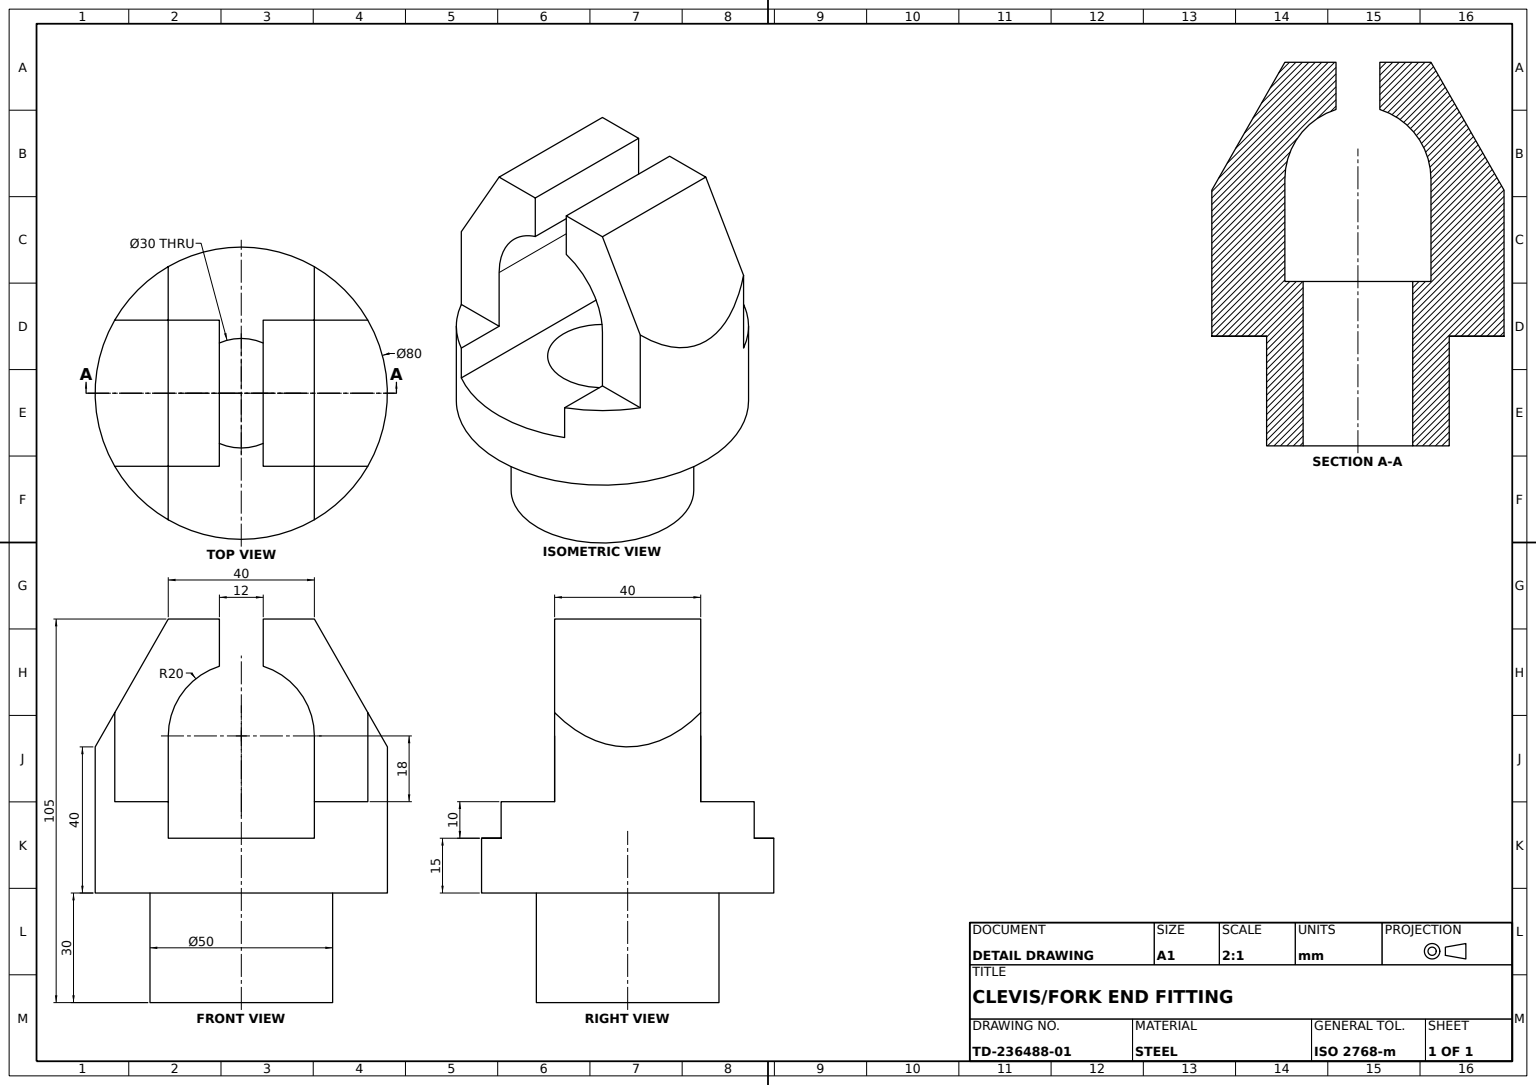
from build123d import *

# Parameters (mm, degrees)
FORK_SIDE_PROFILE_CUT_DEPTH      = 120.268604419
FORK_SIDE_PROFILE_CUT_DEPTH_BACK = 120.268604419
FORK_SIDE_PROFILE_SKETCH_W       = 20
FORK_SIDE_PROFILE_SKETCH_H       = 50
FORK_SLOT_CUT_DEPTH              = 120.268604419
FORK_SLOT_CUT_DEPTH_BACK         = 120.268604419


with BuildPart() as part:
    # Body Profile Sketch → Revolved Body (revolve)
    with BuildSketch(Plane.XY, mode=Mode.PRIVATE) as revolved_body_sk:
        Polygon((15, 0), (25, 0), (25, 30), (40, 30), (40, 105), (0, 105), (0, 55), (15, 55), align=None)
    revolve(revolved_body_sk.sketch.rotate(Axis((0, 0, 0), (0, 1, 0)), 90), axis=Axis((0, 0, 0), (0, 1, 0)))

    # Fork Side Profile Sketch → Fork Side Profile Cut (cut, two sides: drawn at the far end of the back side and taken through both)
    with BuildSketch(Plane(origin=(0, 0, 0), x_dir=(0, 0, -1), z_dir=(1, 0, 0)).offset(-FORK_SIDE_PROFILE_CUT_DEPTH_BACK)):
        with Locations((-30, 80)):
            Rectangle(FORK_SIDE_PROFILE_SKETCH_W, FORK_SIDE_PROFILE_SKETCH_H)
        with Locations((30, 80)):
            Rectangle(FORK_SIDE_PROFILE_SKETCH_W, FORK_SIDE_PROFILE_SKETCH_H)
    extrude(amount=FORK_SIDE_PROFILE_CUT_DEPTH + FORK_SIDE_PROFILE_CUT_DEPTH_BACK, mode=Mode.SUBTRACT)

    # Fork Slot Sketch → Fork Slot Cut (cut, two sides: drawn at the far end of the back side and taken through both)
    with BuildSketch(Plane.XY.offset(-FORK_SLOT_CUT_DEPTH_BACK)):
        Polygon((-40, 105), (-20, 105), (-40, 70), align=None)
        Polygon((40, 105), (20, 105), (40, 70), align=None)
        with BuildLine():
            Line((-20, 45), (20, 45))
            Line((20, 45), (20, 73))
            ThreePointArc((20, 73), (16.124515497, 84.832159566), (6, 92.078784028))
            Line((6, 92.078784028), (6, 105))
            Line((6, 105), (-6, 105))
            Line((-6, 105), (-6, 92.078784028))
            ThreePointArc((-6, 92.078784028), (-16.124515497, 84.832159566), (-20, 73))
            Line((-20, 73), (-20, 45))
        make_face()
    extrude(amount=FORK_SLOT_CUT_DEPTH + FORK_SLOT_CUT_DEPTH_BACK, mode=Mode.SUBTRACT)


solid = part.part
